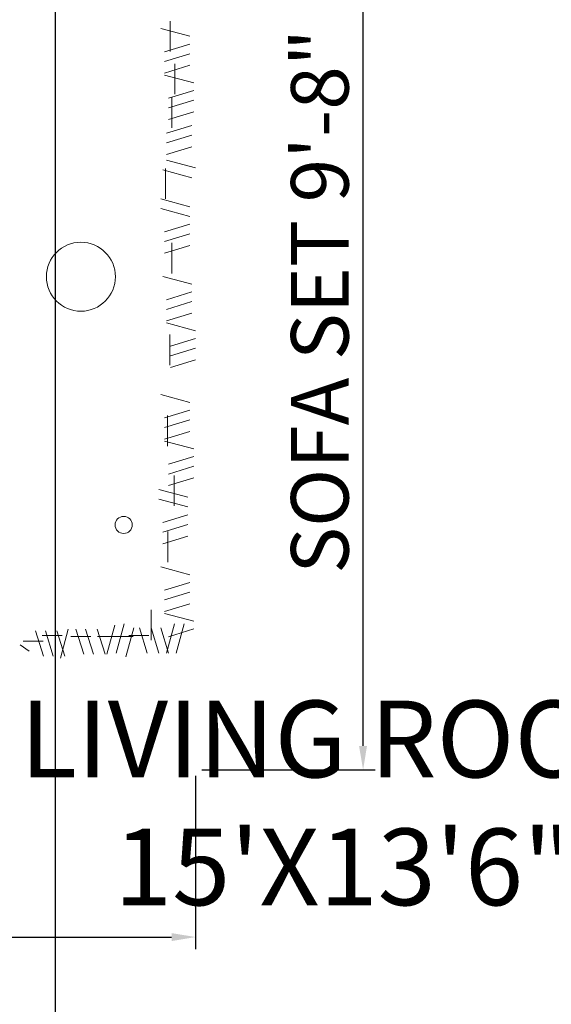
# Model space of a CAD drawing. Units: millimetres. Extents: x 20768 to 23556, y 50760 to 52704.
# Tile 11 of 36: x 20976 to 21032, y 51904 to 52007. Entities that reach past the tile are written whole.
import ezdxf

# ---------------------------------------------------------------- set-up
doc = ezdxf.new("R2010")
doc.units = ezdxf.units.MM
for name, color, linetype, lineweight in [('A-AREA-IDEN', 40, 'Continuous', 18), ('A-FURN', 8, 'Continuous', 18), ('S-ANNO-DIMS', 2, 'Continuous', 18)]:
    doc.layers.add(name, color=color, linetype=linetype, lineweight=lineweight)
doc.styles.get("Standard").update_dxf_attribs({"font": 'arial.ttf'})
doc.dimstyles.new('ISO-25', dxfattribs={"dimtxt": 6, "dimasz": 2.5, "dimexe": 1.25, "dimexo": 0.625, "dimtad": 1, "dimdec": 0, "dimlunit": 3, "dimtxsty": 'Standard', "dimcen": 2.5, "dimadec": 0, "dimazin": 0, "dimtfac": 1, "dimtdec": 0, "dimtmove": 0, "dimatfit": 3, "dimfxl": 1, "dimarcsym": 0})

# ---------------------------------------------------------------- blocks, each defined once
blk = doc.blocks.new('A$C32DD204E')
for p, q in [((2304.1, 2273.8, 685.7), (2304.1, 2181.3, 685.7)), ((2364.1, 2228.1, -685.7), (2275.9, 2251.6, -685.7)), ((2364.1, 2204.5, -685.7), (2287.7, 2181, -685.7)), ((2364.1, 2175.1, -685.7), (2287.7, 2151.6, -685.7)), ((2364.1, 2139.8, -685.7), (2287.7, 2116.3, -685.7)), ((2319.2, 2144.3, 685.7), (2319.2, 2051.7, 685.7)), ((2375.9, 2086.9, -685.7), (2287.7, 2110.4, -685.7)), ((2375.9, 2063.3, -685.7), (2299.4, 2039.8, -685.7)), ((2375.9, 2033.9, -685.7), (2299.4, 2010.4, -685.7)), ((2309.8, 2042.9, 685.7), (2309.8, 1950.3, 685.7)), ((2375.9, 1998.6, -685.7), (2299.4, 1975.1, -685.7)), ((2370, 1957.5, -685.7), (2293.6, 1933.9, -685.7)), ((2370, 1928, -685.7), (2293.6, 1904.5, -685.7)), ((2370, 1892.7, -685.7), (2293.6, 1869.2, -685.7)), ((2290.3, 1826.8, 685.7), (2290.3, 1734.2, 685.7)), ((2381.8, 1828, -685.7), (2293.6, 1851.6, -685.7)), ((2370, 1798.6, -685.7), (2281.8, 1822.1, -685.7)), ((2364.1, 1710.4, -685.7), (2275.9, 1733.9, -685.7)), ((2364.1, 1681, -685.7), (2275.9, 1704.5, -685.7)), ((2364.1, 1657.4, -685.7), (2287.7, 1633.9, -685.7)), ((2364.1, 1628, -685.7), (2287.7, 1604.5, -685.7)), ((2364.1, 1592.7, -685.7), (2287.7, 1569.2, -685.7)), ((2309.8, 1600.2, 685.7), (2309.8, 1507.6, 685.7)), ((2370, 1475.1, -685.7), (2281.8, 1498.6, -685.7)), ((2370, 1451.5, -685.7), (2293.6, 1428, -685.7)), ((2370, 1422.1, -685.7), (2293.6, 1398.6, -685.7)), ((2370, 1386.8, -685.7), (2293.6, 1363.3, -685.7)), ((2381.8, 1333.9, -685.7), (2293.6, 1357.4, -685.7)), ((2303.3, 1321.8, 685.7), (2303.3, 1229.3, 685.7)), ((2381.8, 1310.3, -685.7), (2305.3, 1286.8, -685.7)), ((2381.8, 1280.9, -685.7), (2305.3, 1257.4, -685.7)), ((2381.8, 1245.6, -685.7), (2305.3, 1222.1, -685.7)), ((2364.1, 1116.2, -685.7), (2275.9, 1139.7, -685.7)), ((2364.1, 1092.7, -685.7), (2287.7, 1069.2, -685.7)), ((2364.1, 1063.3, -685.7), (2287.7, 1039.7, -685.7)), ((2296.8, 1075.8, 685.7), (2296.8, 983.2, 685.7)), ((2364.1, 1028, -685.7), (2287.7, 1004.4, -685.7)), ((2375.9, 975, -685.7), (2287.7, 998.6, -685.7)), ((2375.9, 951.5, -685.7), (2299.4, 928, -685.7)), ((2375.9, 922.1, -685.7), (2299.4, 898.6, -685.7)), ((2375.9, 886.8, -685.7), (2299.4, 863.3, -685.7)), ((2316.2, 894.5, 685.7), (2316.2, 802, 685.7)), ((2358.2, 828, -685.7), (2270, 851.5, -685.7)), ((2358.2, 798.5, -685.7), (2270, 822.1, -685.7)), ((2358.2, 775, -685.7), (2281.8, 751.5, -685.7)), ((2358.2, 745.6, -685.7), (2281.8, 722.1, -685.7)), ((2297.3, 723.5, 685.7), (2297.3, 631, 685.7)), ((2358.2, 710.3, -685.7), (2281.8, 686.8, -685.7)), ((2364.1, 592.6, -685.7), (2275.9, 616.2, -685.7)), ((2364.1, 569.1, -685.7), (2287.7, 545.6, -685.7)), ((2364.1, 539.7, -685.7), (2287.7, 516.2, -685.7)), ((2247.2, 486.1, 685.7), (2247.2, 393.6, 685.7)), ((2364.1, 504.4, -685.7), (2287.7, 480.9, -685.7)), ((2375.9, 451.5, -685.7), (2287.7, 475, -685.7)), ((1896.4, 421.9, -685.7), (1920, 345.5, -685.7)), ((1925.8, 421.9, -685.7), (1949.4, 345.5, -685.7)), ((1961.1, 421.9, -685.7), (1984.7, 345.5, -685.7)), ((1995.1, 427.8, -685.7), (1971.6, 339.6, -685.7)), ((2018.7, 427.8, -685.7), (2042.2, 351.4, -685.7)), ((2048.1, 427.8, -685.7), (2071.6, 351.4, -685.7)), ((2083.4, 427.8, -685.7), (2106.9, 351.4, -685.7)), ((2136.3, 439.6, -685.7), (2112.8, 351.4, -685.7)), ((2140.9, 354.9, -685.7), (2164.5, 443.1, -685.7)), ((2170.4, 343.2, -685.7), (2193.9, 431.3, -685.7)), ((2235.1, 354.9, -685.7), (2211.5, 431.3, -685.7)), ((2270.4, 354.9, -685.7), (2246.8, 431.3, -685.7)), ((2299.8, 354.9, -685.7), (2276.2, 431.3, -685.7)), ((2293.8, 354.9, -685.7), (2317.3, 443.1, -685.7)), ((2375.9, 427.9, -685.7), (2299.4, 404.4, -685.7)), ((2323.2, 354.9, -685.7), (2346.7, 443.1, -685.7)), ((1858.6, 391.3), (1919.3, 391.3)), ((1915.9, 408.1), (1976.6, 408.1)), ((2003.6, 404.8), (2064.3, 404.8)), ((2084.5, 404.8), (2145.2, 404.8)), ((2131.7, 404.8), (2192.4, 404.8)), ((2178.9, 408.1), (2239.6, 408.1)), ((1849.9, 380.2, -685.7), (1876.3, 360.8, -685.7))]:
    blk.add_line(p, q)
for centre, radius in [((2033.7, 1497.8, -685.7), 104.7), ((2163.6, 744, -685.7), 26)]:
    blk.add_circle(centre, radius)
blk = doc.blocks.new('*D191')
at = {"layer": 'Defpoints', "color": 0, "transparency": 16777216}
for p in [(20994.76, 52044.82), (21012.2, 52044.82), (20994.76, 51928.59)]:
    blk.add_point(p, dxfattribs=at)
at = {"layer": 'S-ANNO-DIMS', "color": 0, "lineweight": -2, "transparency": 16777216}
for p, q in [((20995.39, 52044.82), (21013.45, 52044.82)), ((21012.2, 51931.09), (21012.2, 52042.32)), ((20995.39, 51928.59), (21013.45, 51928.59))]:
    blk.add_line(p, q, dxfattribs=at)
at = {"layer": 'S-ANNO-DIMS', "color": 0, "transparency": 16777216}
for points in [[(21011.78, 52042.32), (21012.61, 52042.32), (21012.2, 52044.82)], [(21011.78, 51931.09), (21012.61, 51931.09), (21012.2, 51928.59)]]:
    blk.add_solid(points, dxfattribs=at)
at = {"layer": 'S-ANNO-DIMS', "color": 0, "transparency": 16777216, "insert": (21008.47, 51986.71), "char_height": 6, "attachment_point": 5, "rotation": 90}
blk.add_mtext('SOFA SET 9\'-8" TYP.', dxfattribs=at)
blk = doc.blocks.new('*D192')
at = {"layer": 'Defpoints', "color": 0, "transparency": 16777216}
for p in [(20912.98, 51928.59), (20994.76, 51928.59), (20994.76, 51911.16)]:
    blk.add_point(p, dxfattribs=at)
at = {"layer": 'S-ANNO-DIMS', "color": 0, "lineweight": -2, "transparency": 16777216}
for p, q in [((20912.98, 51927.97), (20912.98, 51909.91)), ((20994.76, 51927.97), (20994.76, 51909.91)), ((20915.48, 51911.16), (20992.26, 51911.16))]:
    blk.add_line(p, q, dxfattribs=at)
at = {"layer": 'S-ANNO-DIMS', "color": 0, "transparency": 16777216}
for points in [[(20915.48, 51911.57), (20915.48, 51910.74), (20912.98, 51911.16)], [(20992.26, 51911.57), (20992.26, 51910.74), (20994.76, 51911.16)]]:
    blk.add_solid(points, dxfattribs=at)
at = {"layer": 'S-ANNO-DIMS', "color": 0, "transparency": 16777216, "insert": (20953.87, 51914.85), "char_height": 6, "attachment_point": 5}
blk.add_mtext('6\'-10" TYP.', dxfattribs=at)
blk = doc.blocks.new('*D206')
at = {"layer": 'Defpoints', "color": 0, "transparency": 16777216}
for p in [(20908.14, 52144.9), (20980.14, 52144.9), (20980.14, 51776.4)]:
    blk.add_point(p, dxfattribs=at)
at = {"layer": 'S-ANNO-DIMS', "color": 0, "lineweight": -2, "transparency": 16777216}
for p, q in [((20908.14, 52144.27), (20908.14, 51775.15)), ((20980.14, 52144.27), (20980.14, 51775.15)), ((20910.64, 51776.4), (20977.64, 51776.4))]:
    blk.add_line(p, q, dxfattribs=at)
at = {"layer": 'S-ANNO-DIMS', "color": 0, "transparency": 16777216}
for points in [[(20910.64, 51776.81), (20910.64, 51775.98), (20908.14, 51776.4)], [(20977.64, 51776.81), (20977.64, 51775.98), (20980.14, 51776.4)]]:
    blk.add_solid(points, dxfattribs=at)
at = {"layer": 'S-ANNO-DIMS', "color": 0, "transparency": 16777216, "insert": (20944.14, 51780.09), "char_height": 6, "attachment_point": 5}
blk.add_mtext('6\'-0"', dxfattribs=at)
blk = doc.blocks.new('*D207')
at = {"layer": 'Defpoints', "color": 0, "transparency": 16777216}
for p in [(20908.14, 52080.4), (21070.14, 52080.4), (21070.14, 51776.4)]:
    blk.add_point(p, dxfattribs=at)
at = {"layer": 'S-ANNO-DIMS', "color": 0, "lineweight": -2, "transparency": 16777216}
for p, q in [((20908.14, 52079.77), (20908.14, 51775.15)), ((21070.14, 52079.77), (21070.14, 51775.15)), ((20910.64, 51776.4), (21067.64, 51776.4))]:
    blk.add_line(p, q, dxfattribs=at)
at = {"layer": 'S-ANNO-DIMS', "color": 0, "transparency": 16777216}
for points in [[(20910.64, 51776.81), (20910.64, 51775.98), (20908.14, 51776.4)], [(21067.64, 51776.81), (21067.64, 51775.98), (21070.14, 51776.4)]]:
    blk.add_solid(points, dxfattribs=at)
at = {"layer": 'S-ANNO-DIMS', "color": 0, "transparency": 16777216, "insert": (20989.14, 51780.09), "char_height": 6, "attachment_point": 5}
blk.add_mtext('13\'-6"', dxfattribs=at)

msp = doc.modelspace()

# ---------------------------------------------------------------- block references
at = {"layer": 'A-FURN', "xscale": 0.0343301531987817, "yscale": 0.0343301531987817, "zscale": 0.0343301531987817}
msp.add_blockref('A$C32DD204E', (20912.99, 51928.59, 23.54), dxfattribs=at)

# ---------------------------------------------------------------- texts
at = {"layer": 'A-AREA-IDEN', "insert": (20976.48, 51935.81), "char_height": 8, "attachment_point": 1}
msp.add_mtext_dynamic_manual_height_columns('LIVING ROOM\\P    15\'X13\'6"', width=94.7826, gutter_width=12.5, heights=[0], dxfattribs=at)

# ---------------------------------------------------------------- dimensions: what is measured, and where the dimension line sits
at = {"layer": 'S-ANNO-DIMS'}
for base, p1, p2, picture, middle in [((20980.14, 51776.4), (20908.14, 52144.9), (20980.14, 52144.9), '*D206', (20944.14, 51780.09)), ((21070.14, 51776.4), (20908.14, 52080.4), (21070.14, 52080.4), '*D207', (20989.14, 51780.09))]:
    dim = msp.add_linear_dim(base=base, p1=p1, p2=p2, dimstyle='ISO-25', override={"dimdec": 1, "dimlfac": 1, "dimrnd": 0, "dimzin": 1, "dimdsep": 46, "dimlunit": 4, "dimfrac": 2}, dxfattribs=at)
    dim.commit()
    dim.dimension.update_dxf_attribs({"geometry": picture, "text_midpoint": middle})
dim = msp.add_linear_dim(base=(21012.2, 52044.82), p1=(20994.76, 51928.59), p2=(20994.76, 52044.82), angle=90, text='SOFA SET <> TYP.', dimstyle='ISO-25', override={"dimdec": 1, "dimrnd": 0, "dimzin": 1, "dimlunit": 4, "dimfrac": 2}, dxfattribs=at)
dim.commit()
dim.dimension.update_dxf_attribs({"geometry": '*D191', "text_midpoint": (21008.47, 51986.71)})
dim = msp.add_linear_dim(base=(20994.76, 51911.16), p1=(20912.98, 51928.59), p2=(20994.76, 51928.59), text='<> TYP.', dimstyle='ISO-25', override={"dimdec": 1, "dimrnd": 0, "dimzin": 1, "dimlunit": 4, "dimfrac": 2}, dxfattribs=at)
dim.commit()
dim.dimension.update_dxf_attribs({"geometry": '*D192', "text_midpoint": (20953.87, 51914.85)})

doc.saveas('drawing.dxf')
